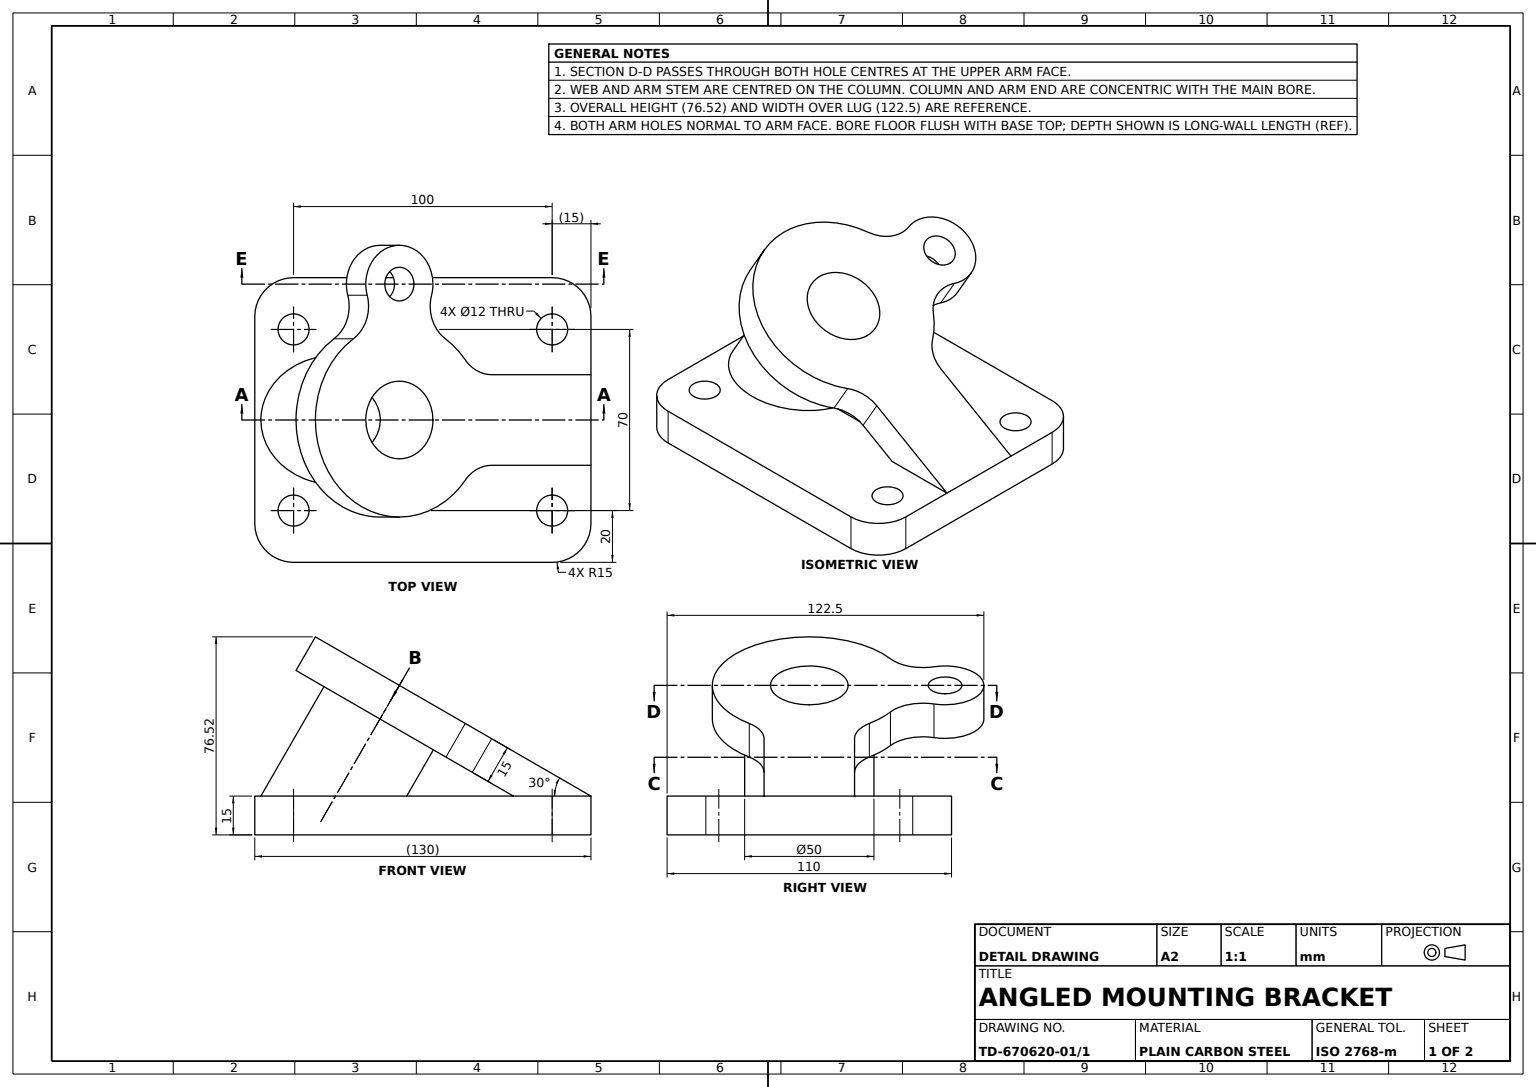
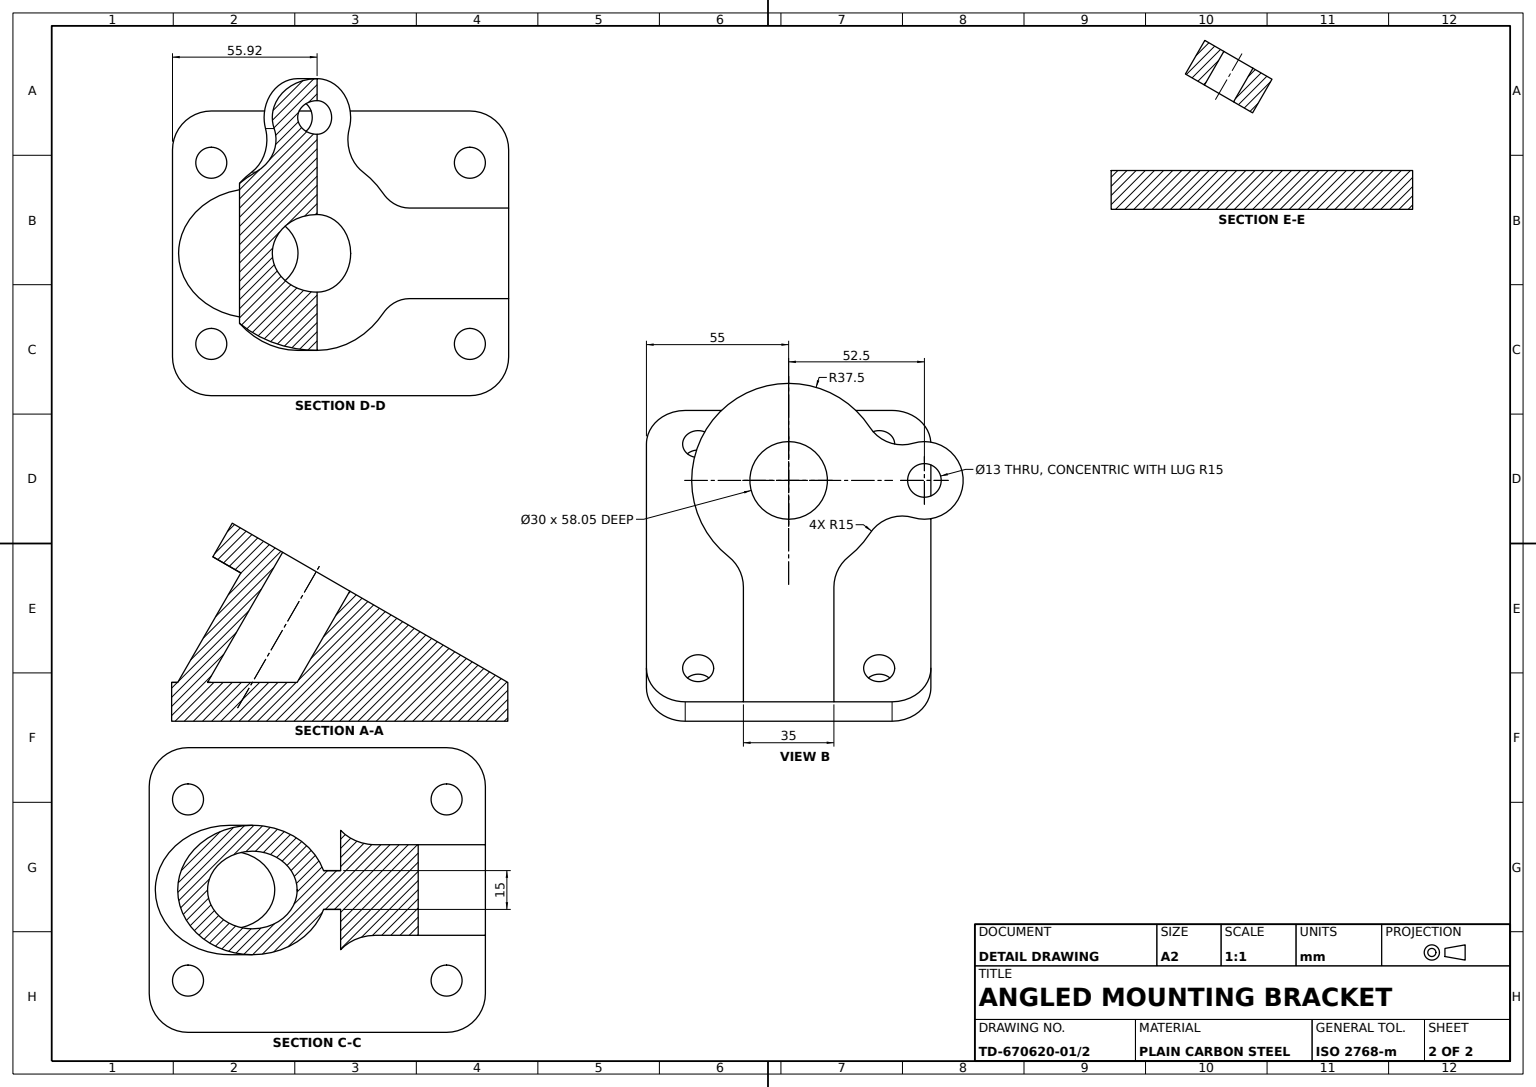
from build123d import *

# Parameters (mm, degrees)
BASE_PLATE_SKETCH_R     = 6
BASE_PLATE_DEPTH        = 15
INCLINED_ARM_SKETCH_R   = 15
INCLINED_ARM_SKETCH_R_2 = 6.5
INCLINED_ARM_DEPTH      = 15
LUG_WITH_BORE_REACH     = 118.221
LUG_SKETCH_R            = 15


with BuildPart() as part:
    # Base Plate Sketch → Base Plate (new body)
    with BuildSketch(Plane(origin=(0, 0, 0), x_dir=(1, 0, 0), z_dir=(0, 1, 0))):
        with BuildLine():
            Line((-50, 55), (50, 55))
            ThreePointArc((50, 55), (60.606601718, 50.606601718), (65, 40))
            Line((65, 40), (65, -40))
            ThreePointArc((65, -40), (60.606601718, -50.606601718), (50, -55))
            Line((50, -55), (-50, -55))
            ThreePointArc((-50, -55), (-60.606601718, -50.606601718), (-65, -40))
            Line((-65, -40), (-65, 40))
            ThreePointArc((-65, 40), (-60.606601718, 50.606601718), (-50, 55))
        make_face()
        with Locations(Location((-50, 35, 0), (0, 0, 270))):
            Circle(BASE_PLATE_SKETCH_R, mode=Mode.SUBTRACT)
        with Locations(Location((-50, -35, 0), (0, 0, 270))):
            Circle(BASE_PLATE_SKETCH_R, mode=Mode.SUBTRACT)
        with Locations(Location((50, -35, 0), (0, 0, 90))):
            Circle(BASE_PLATE_SKETCH_R, mode=Mode.SUBTRACT)
        with Locations(Location((50, 35, 0), (0, 0, 90))):
            Circle(BASE_PLATE_SKETCH_R, mode=Mode.SUBTRACT)
    extrude(amount=BASE_PLATE_DEPTH)

    # Lug Sketch → Lug with Bore (add, up to next)
    with BuildSketch(Plane(origin=(15.245190528, 26.405444566, 0), x_dir=(0.8660254037844417, -0.4999999999999947, 0), z_dir=(-0.4999999999999947, -0.8660254037844417, 0)), mode=Mode.PRIVATE) as lug_with_bore_sk1:
        with BuildLine():
            ThreePointArc((-12.905713736, 7.5), (-61.754193771, 0), (-12.905713736, -7.5))
            Line((-12.905713736, -7.5), (48.791651246, -7.5))
            Line((48.791651246, -7.5), (48.791651246, 7.5))
            Line((48.791651246, 7.5), (-12.905713736, 7.5))
        make_face()
        with Locations(Location((-36.754193771, 0, 0), (0, 0, 180))):
            Circle(LUG_SKETCH_R, mode=Mode.SUBTRACT)
    lug_with_bore_tool1 = extrude(lug_with_bore_sk1.sketch, amount=LUG_WITH_BORE_REACH, mode=Mode.PRIVATE) - part.part


with BuildPart() as body_2:
    # Inclined Arm Sketch → Inclined Arm (new body)
    with BuildSketch(Plane(origin=(22.745190528, 39.395825623, 0), x_dir=(-0.8660254037844417, 0.4999999999999947, 0), z_dir=(0.4999999999999947, 0.8660254037844417, 0))):
        with BuildLine():
            Line((-4.476862485, 17.5), (-48.791651246, 17.5))
            Line((-48.791651246, 17.5), (-48.791651246, -17.5))
            Line((-48.791651246, -17.5), (-4.476862485, -17.5))
            ThreePointArc((-4.476862485, -17.5), (2.069674222, -19.003968837), (7.303439302, -23.214285714))
            ThreePointArc((7.303439302, -23.214285714), (11.430063197, -27.657519966), (16.21887561, -31.37755102))
            ThreePointArc((16.21887561, -31.37755102), (22.091371242, -38.774247477), (22.379471059, -48.214285714))
            ThreePointArc((22.379471059, -48.214285714), (36.754193771, -67.5), (51.128916484, -48.214285714))
            ThreePointArc((51.128916484, -48.214285714), (51.4170163, -38.774247477), (57.289511932, -31.37755102))
            ThreePointArc((57.289511932, -31.37755102), (64.411713737, 25.324130574), (7.303439302, 23.214285714))
            ThreePointArc((7.303439302, 23.214285714), (2.069674222, 19.003968837), (-4.476862485, 17.5))
        make_face()
        with Locations((36.754193771, 0)):
            Circle(INCLINED_ARM_SKETCH_R, mode=Mode.SUBTRACT)
        with Locations((36.754193771, -52.5)):
            Circle(INCLINED_ARM_SKETCH_R_2, mode=Mode.SUBTRACT)
    extrude(amount=-INCLINED_ARM_DEPTH)


with BuildPart() as part_1:
    add(part.part)

    add(body_2.part)  # Lug with Bore merges body 2
    add(lug_with_bore_tool1.solids().sort_by_distance((3.499955, 33.18656, 0))[0])


solid = part_1.part
